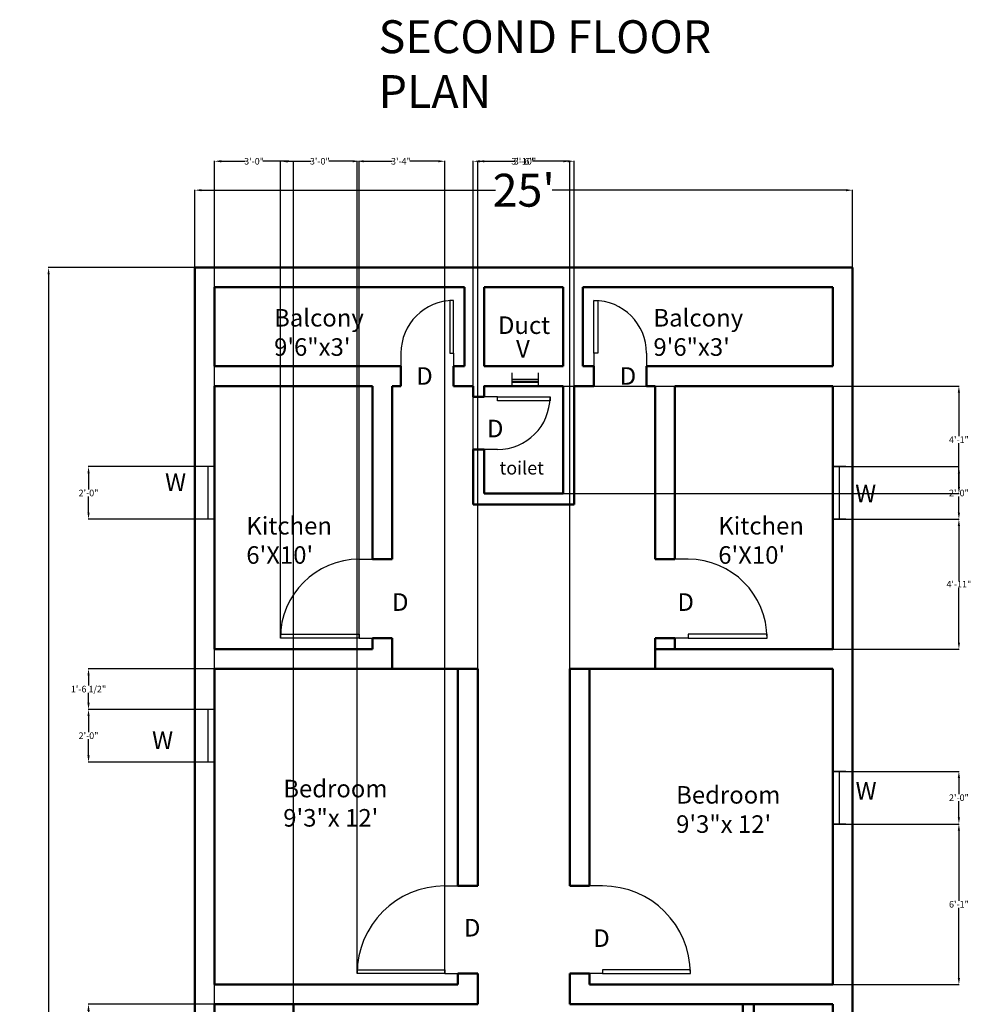
# Model space of a CAD drawing. Units: inches. Extents: x -250 to 2650, y 180 to 1183.
# Tile 6 of 10: x 952 to 1386, y 734 to 1183. Entities that reach past the tile are written whole.
import ezdxf

# ---------------------------------------------------------------- set-up
doc = ezdxf.new("R2010")
doc.units = ezdxf.units.IN
doc.header["$MEASUREMENT"] = 0
for name, color, linetype, lineweight in [('A-ANNO-DIMS', 2, 'Continuous', 18), ('A-ANNO-TEXT', 7, 'Continuous', 18), ('A-AREA-IDEN', 3, 'Continuous', 18), ('A-DOOR', 4, 'Continuous', 25), ('A-GLAZ', 3, 'Continuous', 25), ('A-WALL', 7, 'Continuous', 50)]:
    doc.layers.add(name, color=color, linetype=linetype, lineweight=lineweight)
doc.styles.get("Standard").update_dxf_attribs({"font": 'arial.ttf'})
doc.dimstyles.get("Standard").update_dxf_attribs({"dimtxt": 3, "dimasz": 3, "dimexe": 0.18, "dimexo": 0.0625, "dimgap": 0.09, "dimtad": 0, "dimtih": 1, "dimtoh": 1, "dimdec": 0, "dimzin": 0, "dimdsep": 46, "dimlunit": 3, "dimtxsty": 'Standard', "dimcen": 0.09, "dimadec": 0, "dimazin": 0, "dimtfac": 1, "dimtdec": 0, "dimtofl": 0, "dimtmove": 0, "dimatfit": 3, "dimfxl": 1, "dimtolj": 1, "dimtzin": 0, "dimarcsym": 0})

# ---------------------------------------------------------------- blocks, each defined once
blk = doc.blocks.new('*D34')
at = {"layer": 'A-ANNO-DIMS', "color": 0, "lineweight": -2, "transparency": 16777216}
for p, q in [((1031.71, 1070.09), (1031.71, 1105.5)), ((1034.71, 1105.32), (1168.77, 1105.32)), ((1328.71, 1105.32), (1194.66, 1105.32)), ((1331.71, 1070.09), (1331.71, 1105.5))]:
    blk.add_line(p, q, dxfattribs=at)
at = {"layer": 'A-ANNO-DIMS', "color": 0, "transparency": 16777216}
for points in [[(1034.71, 1105.82), (1034.71, 1104.82), (1031.71, 1105.32)], [(1328.71, 1105.82), (1328.71, 1104.82), (1331.71, 1105.32)]]:
    blk.add_solid(points, dxfattribs=at)
at = {"layer": 'Defpoints', "color": 0, "transparency": 16777216}
for p in [(1031.71, 1105.32), (1031.71, 1070.02), (1331.71, 1070.02)]:
    blk.add_point(p, dxfattribs=at)
at = {"layer": 'A-ANNO-DIMS', "color": 0, "transparency": 16777216, "insert": (1181.71, 1105.32), "char_height": 3, "attachment_point": 5}
blk.add_mtext("\\A1;{\\H5x;25'}", dxfattribs=at)
blk = doc.blocks.new('*D35')
at = {"layer": 'A-ANNO-DIMS', "color": 0, "lineweight": -2, "transparency": 16777216}
for p, q in [((1031.65, 1070.02), (964.83, 1070.02)), ((965.01, 1067.02), (965.01, 657.77)), ((965.01, 233.02), (965.01, 642.28)), ((1031.65, 230.02), (964.83, 230.02))]:
    blk.add_line(p, q, dxfattribs=at)
at = {"layer": 'A-ANNO-DIMS', "color": 0, "transparency": 16777216}
for points in [[(964.51, 1067.02), (965.51, 1067.02), (965.01, 1070.02)], [(964.51, 233.02), (965.51, 233.02), (965.01, 230.02)]]:
    blk.add_solid(points, dxfattribs=at)
at = {"layer": 'Defpoints', "color": 0, "transparency": 16777216}
for p in [(1031.71, 1070.02), (965.01, 230.02), (1031.71, 230.02)]:
    blk.add_point(p, dxfattribs=at)
at = {"layer": 'A-ANNO-DIMS', "color": 0, "transparency": 16777216, "insert": (965.01, 650.02), "char_height": 3, "attachment_point": 5}
blk.add_mtext("\\A1;{\\H5x;70'}", dxfattribs=at)
blk = doc.blocks.new('*U17')
for p, q in [((-24, 0), (-24, -6)), ((0, 0), (0, -6))]:
    blk.add_line(p, q)
blk.add_lwpolyline([(0, 0), (0, 24), (-1.75, 24), (-1.75, 0)], close=True)
blk.add_arc((0, 0), 24, 90, 180)
blk = doc.blocks.new('*U18')
for p, q in [((0, 0), (0, -6)), ((24, 0), (24, -6))]:
    blk.add_line(p, q)
blk.add_lwpolyline([(0, 0), (0, 24), (1.75, 24), (1.75, 0)], close=True)
blk.add_arc((0, 0), 24, 0, 90)
blk = doc.blocks.new('*U19')
for p, q in [((0, 0), (0, -6)), ((24, 0), (24, -6))]:
    blk.add_line(p, q)
blk.add_lwpolyline([(0, 0), (0, 24), (1.75, 24), (1.75, 0)], close=True)
blk.add_arc((0, 0), 24, 0, 90)
blk = doc.blocks.new('*U20')
for p, q in [((-36, 0), (-36, -6)), ((0, 0), (0, -6))]:
    blk.add_line(p, q)
blk.add_lwpolyline([(0, 0), (0, 36), (-1.75, 36), (-1.75, 0)], close=True)
blk.add_arc((0, 0), 36, 90, 180)
blk = doc.blocks.new('*U21')
for p, q in [((-36, 0), (-36, 6)), ((0, 0), (0, 6))]:
    blk.add_line(p, q)
blk.add_lwpolyline([(0, 0), (0, -36), (-1.75, -36), (-1.75, 0)], close=True)
blk.add_arc((0, 0), 36, 180, 270)
blk = doc.blocks.new('*U24')
for p, q in [((-24, 6), (-24, 0)), ((0, 6), (0, 0)), ((0, 3), (-24, 3))]:
    blk.add_line(p, q)
blk = doc.blocks.new('*U23')
for p, q in [((-24, 6), (-24, 0)), ((0, 6), (0, 0)), ((0, 3), (-24, 3))]:
    blk.add_line(p, q)
blk = doc.blocks.new('*U22')
for p, q in [((0, 6), (0, 0)), ((12, 6), (12, 0)), ((0, 3), (12, 3))]:
    blk.add_line(p, q)
blk = doc.blocks.new('*U25')
for p, q in [((-40, 0), (-40, 6)), ((0, 0), (0, 6))]:
    blk.add_line(p, q)
blk.add_lwpolyline([(0, 0), (0, -40), (-1.75, -40), (-1.75, 0)], close=True)
blk.add_arc((0, 0), 40, 180, 270)
blk = doc.blocks.new('*U26')
for p, q in [((-40, 0), (-40, -6)), ((0, 0), (0, -6))]:
    blk.add_line(p, q)
blk.add_lwpolyline([(0, 0), (0, 40), (-1.75, 40), (-1.75, 0)], close=True)
blk.add_arc((0, 0), 40, 90, 180)
blk = doc.blocks.new('*D112')
at = {"layer": 'A-ANNO-DIMS', "color": 0, "lineweight": -2, "transparency": 16777216}
for p, q in [((1040.71, 734.09), (1040.71, 1118.7)), ((1043.71, 1118.52), (1054.64, 1118.52)), ((1073.71, 1118.52), (1062.79, 1118.52)), ((1076.71, 734.09), (1076.71, 1118.7))]:
    blk.add_line(p, q, dxfattribs=at)
at = {"layer": 'A-ANNO-DIMS', "color": 0, "transparency": 16777216}
for points in [[(1043.71, 1119.02), (1043.71, 1118.02), (1040.71, 1118.52)], [(1073.71, 1119.02), (1073.71, 1118.02), (1076.71, 1118.52)]]:
    blk.add_solid(points, dxfattribs=at)
at = {"layer": 'Defpoints', "color": 0, "transparency": 16777216}
for p in [(1076.71, 1118.52), (1040.71, 734.02), (1076.71, 734.02)]:
    blk.add_point(p, dxfattribs=at)
at = {"layer": 'A-ANNO-DIMS', "color": 0, "transparency": 16777216, "insert": (1058.71, 1118.52), "char_height": 3, "attachment_point": 5}
blk.add_mtext('\\A1;3\'-0"', dxfattribs=at)
blk = doc.blocks.new('*D114')
at = {"layer": 'A-ANNO-DIMS', "color": 0, "lineweight": -2, "transparency": 16777216}
for p, q in [((1040.65, 734.02), (983.03, 734.02)), ((983.21, 731.02), (983.21, 717.09)), ((983.21, 699.91), (983.21, 713.84)), ((1040.65, 696.91), (983.03, 696.91))]:
    blk.add_line(p, q, dxfattribs=at)
at = {"layer": 'A-ANNO-DIMS', "color": 0, "transparency": 16777216}
for points in [[(982.71, 731.02), (983.71, 731.02), (983.21, 734.02)], [(982.71, 699.91), (983.71, 699.91), (983.21, 696.91)]]:
    blk.add_solid(points, dxfattribs=at)
at = {"layer": 'Defpoints', "color": 0, "transparency": 16777216}
for p in [(983.21, 734.02), (1040.71, 734.02), (1040.71, 696.91)]:
    blk.add_point(p, dxfattribs=at)
at = {"layer": 'A-ANNO-DIMS', "color": 0, "transparency": 16777216, "insert": (983.21, 715.47), "char_height": 3, "attachment_point": 5}
blk.add_mtext('\\A1;3\'-1"', dxfattribs=at)
blk = doc.blocks.new('*D122')
at = {"layer": 'A-ANNO-DIMS', "color": 0, "lineweight": -2, "transparency": 16777216}
for p, q in [((1160.71, 887.09), (1160.71, 1118.7)), ((1163.71, 1118.52), (1177.64, 1118.52)), ((1199.71, 1118.52), (1185.79, 1118.52)), ((1202.71, 887.09), (1202.71, 1118.7))]:
    blk.add_line(p, q, dxfattribs=at)
at = {"layer": 'A-ANNO-DIMS', "color": 0, "transparency": 16777216}
for points in [[(1163.71, 1119.02), (1163.71, 1118.02), (1160.71, 1118.52)], [(1199.71, 1119.02), (1199.71, 1118.02), (1202.71, 1118.52)]]:
    blk.add_solid(points, dxfattribs=at)
at = {"layer": 'Defpoints', "color": 0, "transparency": 16777216}
for p in [(1202.71, 1118.52), (1160.71, 887.02), (1202.71, 887.02)]:
    blk.add_point(p, dxfattribs=at)
at = {"layer": 'A-ANNO-DIMS', "color": 0, "transparency": 16777216, "insert": (1181.71, 1118.52), "char_height": 3, "attachment_point": 5}
blk.add_mtext('\\A1;3\'-6"', dxfattribs=at)
blk = doc.blocks.new('*D123')
at = {"layer": 'A-ANNO-DIMS', "color": 0, "lineweight": -2, "transparency": 16777216}
for p, q in [((1158.71, 962.09), (1158.71, 1118.7)), ((1161.71, 1118.52), (1176.47, 1118.52)), ((1201.71, 1118.52), (1186.96, 1118.52)), ((1204.71, 962.09), (1204.71, 1118.7))]:
    blk.add_line(p, q, dxfattribs=at)
at = {"layer": 'A-ANNO-DIMS', "color": 0, "transparency": 16777216}
for points in [[(1161.71, 1119.02), (1161.71, 1118.02), (1158.71, 1118.52)], [(1201.71, 1119.02), (1201.71, 1118.02), (1204.71, 1118.52)]]:
    blk.add_solid(points, dxfattribs=at)
at = {"layer": 'Defpoints', "color": 0, "transparency": 16777216}
for p in [(1204.71, 1118.52), (1158.71, 962.02), (1204.71, 962.02)]:
    blk.add_point(p, dxfattribs=at)
at = {"layer": 'A-ANNO-DIMS', "color": 0, "transparency": 16777216, "insert": (1181.71, 1118.52), "char_height": 3, "attachment_point": 5}
blk.add_mtext('\\A1;3\'-10"', dxfattribs=at)
blk = doc.blocks.new('*D124')
at = {"layer": 'A-ANNO-DIMS', "color": 0, "lineweight": -2, "transparency": 16777216}
for p, q in [((1199.78, 1016.02), (1380.39, 1016.02)), ((1380.21, 1013.02), (1380.21, 993.12)), ((1380.21, 970.02), (1380.21, 989.93)), ((1199.78, 967.02), (1380.39, 967.02))]:
    blk.add_line(p, q, dxfattribs=at)
at = {"layer": 'A-ANNO-DIMS', "color": 0, "transparency": 16777216}
for points in [[(1379.71, 1013.02), (1380.71, 1013.02), (1380.21, 1016.02)], [(1379.71, 970.02), (1380.71, 970.02), (1380.21, 967.02)]]:
    blk.add_solid(points, dxfattribs=at)
at = {"layer": 'Defpoints', "color": 0, "transparency": 16777216}
for p in [(1199.71, 1016.02), (1199.71, 967.02), (1380.21, 967.02)]:
    blk.add_point(p, dxfattribs=at)
at = {"layer": 'A-ANNO-DIMS', "color": 0, "transparency": 16777216, "insert": (1380.21, 991.52), "char_height": 3, "attachment_point": 5}
blk.add_mtext('\\A1;4\'-1"', dxfattribs=at)
blk = doc.blocks.new('*D125')
at = {"layer": 'A-ANNO-DIMS', "color": 0, "lineweight": -2, "transparency": 16777216}
for p, q in [((1322.78, 816.25), (1380.39, 816.25)), ((1380.21, 813.25), (1380.21, 781.26)), ((1380.21, 746.02), (1380.21, 778.01)), ((1322.78, 743.02), (1380.39, 743.02))]:
    blk.add_line(p, q, dxfattribs=at)
at = {"layer": 'A-ANNO-DIMS', "color": 0, "transparency": 16777216}
for points in [[(1379.71, 813.25), (1380.71, 813.25), (1380.21, 816.25)], [(1379.71, 746.02), (1380.71, 746.02), (1380.21, 743.02)]]:
    blk.add_solid(points, dxfattribs=at)
at = {"layer": 'Defpoints', "color": 0, "transparency": 16777216}
for p in [(1322.71, 816.25), (1380.21, 816.25), (1322.71, 743.02)]:
    blk.add_point(p, dxfattribs=at)
at = {"layer": 'A-ANNO-DIMS', "color": 0, "transparency": 16777216, "insert": (1380.21, 779.64), "char_height": 3, "attachment_point": 5}
blk.add_mtext('\\A1;6\'-1"', dxfattribs=at)
blk = doc.blocks.new('*D126')
at = {"layer": 'A-ANNO-DIMS', "color": 0, "lineweight": -2, "transparency": 16777216}
for p, q in [((1322.78, 840.25), (1380.39, 840.25)), ((1380.21, 837.25), (1380.21, 829.87)), ((1380.21, 819.25), (1380.21, 826.63)), ((1322.78, 816.25), (1380.39, 816.25))]:
    blk.add_line(p, q, dxfattribs=at)
at = {"layer": 'A-ANNO-DIMS', "color": 0, "transparency": 16777216}
for points in [[(1379.71, 837.25), (1380.71, 837.25), (1380.21, 840.25)], [(1379.71, 819.25), (1380.71, 819.25), (1380.21, 816.25)]]:
    blk.add_solid(points, dxfattribs=at)
at = {"layer": 'Defpoints', "color": 0, "transparency": 16777216}
for p in [(1322.71, 840.25), (1380.21, 840.25), (1322.71, 816.25)]:
    blk.add_point(p, dxfattribs=at)
at = {"layer": 'A-ANNO-DIMS', "color": 0, "transparency": 16777216, "insert": (1380.21, 828.25), "char_height": 3, "attachment_point": 5}
blk.add_mtext('\\A1;2\'-0"', dxfattribs=at)
blk = doc.blocks.new('*D127')
at = {"layer": 'A-ANNO-DIMS', "color": 0, "lineweight": -2, "transparency": 16777216}
for p, q in [((1322.78, 955.23), (1380.39, 955.23)), ((1380.21, 952.23), (1380.21, 927.22)), ((1380.21, 899.02), (1380.21, 924.03)), ((1322.78, 896.02), (1380.39, 896.02))]:
    blk.add_line(p, q, dxfattribs=at)
at = {"layer": 'A-ANNO-DIMS', "color": 0, "transparency": 16777216}
for points in [[(1379.71, 952.23), (1380.71, 952.23), (1380.21, 955.23)], [(1379.71, 899.02), (1380.71, 899.02), (1380.21, 896.02)]]:
    blk.add_solid(points, dxfattribs=at)
at = {"layer": 'Defpoints', "color": 0, "transparency": 16777216}
for p in [(1322.71, 955.23), (1380.21, 955.23), (1322.71, 896.02)]:
    blk.add_point(p, dxfattribs=at)
at = {"layer": 'A-ANNO-DIMS', "color": 0, "transparency": 16777216, "insert": (1380.21, 925.63), "char_height": 3, "attachment_point": 5}
blk.add_mtext('\\A1;4\'-11"', dxfattribs=at)
blk = doc.blocks.new('*D128')
at = {"layer": 'A-ANNO-DIMS', "color": 0, "lineweight": -2, "transparency": 16777216}
for p, q in [((1322.78, 979.23), (1380.39, 979.23)), ((1380.21, 976.23), (1380.21, 968.85)), ((1380.21, 958.23), (1380.21, 965.61)), ((1322.78, 955.23), (1380.39, 955.23))]:
    blk.add_line(p, q, dxfattribs=at)
at = {"layer": 'A-ANNO-DIMS', "color": 0, "transparency": 16777216}
for points in [[(1379.71, 976.23), (1380.71, 976.23), (1380.21, 979.23)], [(1379.71, 958.23), (1380.71, 958.23), (1380.21, 955.23)]]:
    blk.add_solid(points, dxfattribs=at)
at = {"layer": 'Defpoints', "color": 0, "transparency": 16777216}
for p in [(1322.71, 979.23), (1380.21, 979.23), (1322.71, 955.23)]:
    blk.add_point(p, dxfattribs=at)
at = {"layer": 'A-ANNO-DIMS', "color": 0, "transparency": 16777216, "insert": (1380.21, 967.23), "char_height": 3, "attachment_point": 5}
blk.add_mtext('\\A1;2\'-0"', dxfattribs=at)
blk = doc.blocks.new('*D129')
at = {"layer": 'A-ANNO-DIMS', "color": 0, "lineweight": -2, "transparency": 16777216}
for p, q in [((1040.65, 868.53), (983.03, 868.53)), ((983.21, 865.53), (983.21, 858.15)), ((983.21, 847.53), (983.21, 854.91)), ((1040.65, 844.53), (983.03, 844.53))]:
    blk.add_line(p, q, dxfattribs=at)
at = {"layer": 'A-ANNO-DIMS', "color": 0, "transparency": 16777216}
for points in [[(982.71, 865.53), (983.71, 865.53), (983.21, 868.53)], [(982.71, 847.53), (983.71, 847.53), (983.21, 844.53)]]:
    blk.add_solid(points, dxfattribs=at)
at = {"layer": 'Defpoints', "color": 0, "transparency": 16777216}
for p in [(983.21, 868.53), (1040.71, 868.53), (1040.71, 844.53)]:
    blk.add_point(p, dxfattribs=at)
at = {"layer": 'A-ANNO-DIMS', "color": 0, "transparency": 16777216, "insert": (983.21, 856.53), "char_height": 3, "attachment_point": 5}
blk.add_mtext('\\A1;2\'-0"', dxfattribs=at)
blk = doc.blocks.new('*D130')
at = {"layer": 'A-ANNO-DIMS', "color": 0, "lineweight": -2, "transparency": 16777216}
for p, q in [((1040.65, 887.02), (983.03, 887.02)), ((983.21, 884.02), (983.21, 879.42)), ((983.21, 871.53), (983.21, 876.14)), ((1040.65, 868.53), (983.03, 868.53))]:
    blk.add_line(p, q, dxfattribs=at)
at = {"layer": 'A-ANNO-DIMS', "color": 0, "transparency": 16777216}
for points in [[(982.71, 884.02), (983.71, 884.02), (983.21, 887.02)], [(982.71, 871.53), (983.71, 871.53), (983.21, 868.53)]]:
    blk.add_solid(points, dxfattribs=at)
at = {"layer": 'Defpoints', "color": 0, "transparency": 16777216}
for p in [(983.21, 887.02), (1040.71, 887.02), (1040.71, 868.53)]:
    blk.add_point(p, dxfattribs=at)
at = {"layer": 'A-ANNO-DIMS', "color": 0, "transparency": 16777216, "insert": (983.21, 877.78), "char_height": 3, "attachment_point": 5}
blk.add_mtext('\\A1;1\'-6 1/2"', dxfattribs=at)
blk = doc.blocks.new('*D131')
at = {"layer": 'A-ANNO-DIMS', "color": 0, "lineweight": -2, "transparency": 16777216}
for p, q in [((1040.65, 979.23), (983.03, 979.23)), ((983.21, 976.23), (983.21, 968.85)), ((983.21, 958.23), (983.21, 965.61)), ((1040.65, 955.23), (983.03, 955.23))]:
    blk.add_line(p, q, dxfattribs=at)
at = {"layer": 'A-ANNO-DIMS', "color": 0, "transparency": 16777216}
for points in [[(982.71, 976.23), (983.71, 976.23), (983.21, 979.23)], [(982.71, 958.23), (983.71, 958.23), (983.21, 955.23)]]:
    blk.add_solid(points, dxfattribs=at)
at = {"layer": 'Defpoints', "color": 0, "transparency": 16777216}
for p in [(983.21, 979.23), (1040.71, 979.23), (1040.71, 955.23)]:
    blk.add_point(p, dxfattribs=at)
at = {"layer": 'A-ANNO-DIMS', "color": 0, "transparency": 16777216, "insert": (983.21, 967.23), "char_height": 3, "attachment_point": 5}
blk.add_mtext('\\A1;2\'-0"', dxfattribs=at)
blk = doc.blocks.new('*D132')
at = {"layer": 'A-ANNO-DIMS', "color": 0, "lineweight": -2, "transparency": 16777216}
for p, q in [((1105.71, 748.09), (1105.71, 1118.7)), ((1108.71, 1118.52), (1121.64, 1118.52)), ((1142.71, 1118.52), (1129.79, 1118.52)), ((1145.71, 748.09), (1145.71, 1118.7))]:
    blk.add_line(p, q, dxfattribs=at)
at = {"layer": 'A-ANNO-DIMS', "color": 0, "transparency": 16777216}
for points in [[(1108.71, 1119.02), (1108.71, 1118.02), (1105.71, 1118.52)], [(1142.71, 1119.02), (1142.71, 1118.02), (1145.71, 1118.52)]]:
    blk.add_solid(points, dxfattribs=at)
at = {"layer": 'Defpoints', "color": 0, "transparency": 16777216}
for p in [(1145.71, 1118.52), (1105.71, 748.02), (1145.71, 748.02)]:
    blk.add_point(p, dxfattribs=at)
at = {"layer": 'A-ANNO-DIMS', "color": 0, "transparency": 16777216, "insert": (1125.71, 1118.52), "char_height": 3, "attachment_point": 5}
blk.add_mtext('\\A1;3\'-4"', dxfattribs=at)
blk = doc.blocks.new('*D133')
at = {"layer": 'A-ANNO-DIMS', "color": 0, "lineweight": -2, "transparency": 16777216}
for p, q in [((1070.71, 901.09), (1070.71, 1118.7)), ((1073.71, 1118.52), (1084.64, 1118.52)), ((1103.71, 1118.52), (1092.79, 1118.52)), ((1106.71, 901.09), (1106.71, 1118.7))]:
    blk.add_line(p, q, dxfattribs=at)
at = {"layer": 'A-ANNO-DIMS', "color": 0, "transparency": 16777216}
for points in [[(1073.71, 1119.02), (1073.71, 1118.02), (1070.71, 1118.52)], [(1103.71, 1119.02), (1103.71, 1118.02), (1106.71, 1118.52)]]:
    blk.add_solid(points, dxfattribs=at)
at = {"layer": 'Defpoints', "color": 0, "transparency": 16777216}
for p in [(1106.71, 1118.52), (1070.71, 901.02), (1106.71, 901.02)]:
    blk.add_point(p, dxfattribs=at)
at = {"layer": 'A-ANNO-DIMS', "color": 0, "transparency": 16777216, "insert": (1088.71, 1118.52), "char_height": 3, "attachment_point": 5}
blk.add_mtext('\\A1;3\'-0"', dxfattribs=at)

msp = doc.modelspace()

# ---------------------------------------------------------------- linework, layer by layer
at = {"layer": 'A-WALL'}
for p, q in [((1331.71, 1070.02), (1031.71, 1070.02)), ((1031.71, 1070.02), (1031.71, 230.02)), ((1331.71, 230.02), (1331.71, 1070.02)), ((1154.71, 1061.02), (1040.71, 1061.02)), ((1040.71, 1061.02), (1040.71, 1025.02)), ((1154.71, 1061.02), (1154.71, 1025.02)), ((1199.71, 1061.02), (1163.71, 1061.02)), ((1163.71, 1061.02), (1163.71, 1025.02)), ((1199.71, 1025.02), (1199.71, 1061.02)), ((1208.71, 1025.02), (1208.71, 1061.02)), ((1322.71, 1061.02), (1208.71, 1061.02)), ((1322.71, 1025.02), (1322.71, 1061.02)), ((1322.71, 1025.02), (1322.71, 1061.02)), ((1322.71, 1025.02), (1322.71, 1061.02)), ((1322.71, 1025.02), (1322.71, 1061.02)), ((1125.71, 1025.02), (1040.71, 1025.02)), ((1125.71, 1025.02), (1125.71, 1016.02)), ((1154.71, 1025.02), (1149.71, 1025.02)), ((1149.71, 1016.02), (1149.71, 1025.02)), ((1199.71, 1025.02), (1163.71, 1025.02)), ((1213.71, 1025.02), (1208.71, 1025.02)), ((1213.71, 1016.02), (1213.71, 1025.02)), ((1322.71, 1025.02), (1237.71, 1025.02)), ((1237.71, 1025.02), (1237.71, 1016.02)), ((1112.71, 1016.02), (1040.71, 1016.02)), ((1040.71, 1016.02), (1040.71, 896.02)), ((1112.71, 1016.02), (1112.71, 937.02)), ((1125.71, 1016.02), (1121.71, 1016.02)), ((1121.71, 1016.02), (1121.71, 937.02)), ((1158.71, 1016.02), (1149.71, 1016.02)), ((1158.71, 1016.02), (1158.71, 1011.02)), ((1163.71, 1016.03), (1163.71, 1011.02)), ((1199.71, 1016.02), (1163.71, 1016.02)), ((1188.4, 1017.95), (1176.4, 1017.95)), ((1199.71, 967.02), (1199.71, 1016.02)), ((1204.71, 962.02), (1204.71, 1016.02)), ((1213.71, 1016.02), (1204.71, 1016.02)), ((1241.71, 1016.02), (1237.71, 1016.02)), ((1241.71, 937.02), (1241.71, 1016.02)), ((1250.71, 937.02), (1250.71, 1016.02)), ((1322.71, 1016.02), (1250.71, 1016.02)), ((1322.71, 896.02), (1322.71, 1016.02)), ((1322.71, 896.02), (1322.71, 1016.02)), ((1322.71, 896.02), (1322.71, 1016.02)), ((1163.71, 1011.02), (1158.71, 1011.02)), ((1158.71, 987.02), (1158.71, 962.02)), ((1163.71, 987.02), (1158.71, 987.02)), ((1163.71, 987.02), (1163.71, 967.02)), ((1199.71, 967.02), (1163.71, 967.02)), ((1204.71, 962.02), (1158.71, 962.02)), ((1112.71, 937.02), (1121.71, 937.02)), ((1250.71, 937.02), (1241.71, 937.02)), ((1112.71, 901.02), (1112.71, 896.02)), ((1112.71, 901.02), (1121.71, 901.02)), ((1121.71, 901.02), (1121.71, 887.02)), ((1241.71, 887.02), (1241.71, 901.02)), ((1250.71, 901.02), (1241.71, 901.02)), ((1250.71, 896.02), (1250.71, 901.02)), ((1112.71, 896.02), (1040.71, 896.02)), ((1322.71, 896.02), (1241.71, 896.02)), ((1160.71, 887.02), (1040.71, 887.02)), ((1040.71, 887.02), (1040.71, 743.02)), ((1151.71, 887.02), (1151.71, 788.02)), ((1160.71, 887.02), (1160.71, 788.02)), ((1202.71, 788.02), (1202.71, 887.02)), ((1322.71, 887.02), (1202.71, 887.02)), ((1211.71, 788.02), (1211.71, 887.02)), ((1322.71, 743.02), (1322.71, 887.02)), ((1322.71, 743.02), (1322.71, 887.02)), ((1322.71, 743.02), (1322.71, 887.02)), ((1151.71, 788.02), (1160.71, 788.02)), ((1211.71, 788.02), (1202.71, 788.02)), ((1151.71, 748.02), (1151.71, 743.02)), ((1151.71, 748.02), (1160.71, 748.02)), ((1160.71, 748.02), (1160.71, 734.02)), ((1211.71, 748.02), (1202.71, 748.02)), ((1202.71, 748.02), (1202.71, 734.02)), ((1211.71, 743.02), (1211.71, 748.02)), ((1151.71, 743.02), (1040.71, 743.02)), ((1322.71, 743.02), (1211.71, 743.02)), ((1160.71, 734.02), (1040.71, 734.02)), ((1040.71, 734.02), (1040.71, 696.91)), ((1076.71, 696.91), (1076.71, 734.02)), ((1322.71, 734.02), (1202.71, 734.02)), ((1281.71, 686.91), (1281.71, 734.02)), ((1281.71, 686.91), (1281.71, 734.02)), ((1286.71, 696.91), (1286.71, 734.02)), ((1322.71, 696.91), (1322.71, 734.02)), ((1322.71, 716.02), (1322.71, 734.02))]:
    msp.add_line(p, q, dxfattribs=at)

# ---------------------------------------------------------------- block references
at = {"layer": 'A-DOOR'}
for name, p in [('*U17', (1149.71, 1031.02)), ('*U18', (1213.71, 1031.02))]:
    msp.add_blockref(name, p, dxfattribs=at)
at = {"layer": 'A-DOOR', "rotation": 270}
for name, p in [('*U19', (1169.71, 1011.02)), ('*U21', (1106.71, 901.02)), ('*U20', (1256.71, 901.02)), ('*U25', (1145.71, 748.02)), ('*U26', (1217.71, 748.02))]:
    msp.add_blockref(name, p, dxfattribs=at)
at = {"layer": 'A-GLAZ'}
for name, p, rotation in [('*U22', (1188.4, 1021.95), 180), ('*U23', (1034.71, 955.23), 270), ('*U24', (1322.71, 955.23), 270), ('*U23', (1034.71, 844.53), 270), ('*U24', (1322.71, 816.25), 270)]:
    msp.add_blockref(name, p, dxfattribs=dict(at, rotation=rotation))

# ---------------------------------------------------------------- texts
at = {"layer": 'A-ANNO-TEXT', "attachment_point": 1}
for s, width, insert, char_height in [('SECOND FLOOR PLAN ', 207.4062, (1115.52, 1182.82), 15), ('V', 10.3916, (1178.22, 1036.98), 8), ('D', 10.3916, (1132.7, 1024.6), 8), ('D', 10.3916, (1225.51, 1024.6), 8), ('D', 10.3916, (1164.95, 1000.62), 8), ('W', 10.3916, (1018.13, 976.14), 8), ('W', 10.3916, (1332.9, 971.03), 8), ('D', 10.3916, (1121.66, 921.46), 8), ('D', 10.3916, (1251.84, 921.46), 8), ('W', 10.3916, (1012.2, 858.45), 8), ('W', 10.3916, (1333.08, 835.41), 8), ('D', 10.3916, (1154.45, 772.95), 8), ('D', 10.3916, (1213.44, 768.2), 8)]:
    msp.add_mtext_dynamic_manual_height_columns(s, width=width, gutter_width=1, heights=[0], dxfattribs=dict(at, insert=insert, char_height=char_height))
at = {"layer": 'A-AREA-IDEN', "attachment_point": 1}
for s, width, heights, insert, char_height in [('Balcony 9\'6"x3\'', 37.1044, [0], (1067.85, 1051.13), 8), ('Balcony 9\'6"x3\'', 37.1044, [0], (1240.87, 1051.13), 8), ('{\\H2.66667x;Duct} ', 7.71, [3.05], (1169.97, 1047.76), 3), ('toilet', 19.3499, [0], (1170.68, 981.65), 6), ("Kitchen 6'X10'", 37.1044, [0], (1055.18, 956.28), 8), ("Kitchen 6'X10'", 37.1044, [0], (1270.45, 956.28), 8), ('Bedroom \\P9\'3"x 12\'', 51.3886, [0], (1072.03, 836.41), 8), ('Bedroom \\P9\'3"x 12\'', 51.3886, [0], (1251.23, 833.56), 8)]:
    msp.add_mtext_dynamic_manual_height_columns(s, width=width, gutter_width=1, heights=heights, dxfattribs=dict(at, insert=insert, char_height=char_height))

# ---------------------------------------------------------------- dimensions: what is measured, and where the dimension line sits
at = {"layer": 'A-ANNO-DIMS'}
for base, p1, p2, picture, middle in [((1076.71, 1118.52), (1040.71, 734.02), (1076.71, 734.02), '*D112', (1058.71, 1118.52)), ((1106.71, 1118.52), (1070.71, 901.02), (1106.71, 901.02), '*D133', (1088.71, 1118.52)), ((1145.71, 1118.52), (1105.71, 748.02), (1145.71, 748.02), '*D132', (1125.71, 1118.52)), ((1204.71, 1118.52), (1158.71, 962.02), (1204.71, 962.02), '*D123', (1181.71, 1118.52)), ((1202.71, 1118.52), (1160.71, 887.02), (1202.71, 887.02), '*D122', (1181.71, 1118.52))]:
    dim = msp.add_linear_dim(base=base, p1=p1, p2=p2, dimstyle='Standard', override={"dimdec": 1, "dimlfac": 1, "dimrnd": 0, "dimzin": 1, "dimdsep": 46, "dimlunit": 4, "dimfrac": 2}, dxfattribs=at)
    dim.commit()
    dim.dimension.update_dxf_attribs({"geometry": picture, "text_midpoint": middle})
dim = msp.add_linear_dim(base=(1031.71, 1105.32), p1=(1331.71, 1070.02), p2=(1031.71, 1070.02), text='{\\H5x;<>}', dimstyle='Standard', override={"dimclrd": 0, "dimclre": 0, "dimclrt": 0}, dxfattribs=at)
dim.commit()
dim.dimension.update_dxf_attribs({"geometry": '*D34', "text_midpoint": (1181.71, 1105.32)})
dim = msp.add_linear_dim(base=(965.01, 230.02), p1=(1031.71, 1070.02), p2=(1031.71, 230.02), angle=90, text='{\\H5x;<>}', dimstyle='Standard', override={"dimclrd": 0, "dimclre": 0, "dimclrt": 0}, dxfattribs=at)
dim.commit()
dim.dimension.update_dxf_attribs({"geometry": '*D35', "text_midpoint": (965.01, 650.02)})
for base, p1, p2, picture, middle in [((1380.21, 967.02), (1199.71, 1016.02), (1199.71, 967.02), '*D124', (1380.21, 991.52)), ((983.21, 979.23), (1040.71, 955.23), (1040.71, 979.23), '*D131', (983.21, 967.23)), ((1380.21, 979.23), (1322.71, 955.23), (1322.71, 979.23), '*D128', (1380.21, 967.23)), ((1380.21, 955.23), (1322.71, 896.02), (1322.71, 955.23), '*D127', (1380.21, 925.63)), ((983.21, 887.02), (1040.71, 868.53), (1040.71, 887.02), '*D130', (983.21, 877.78)), ((983.21, 868.53), (1040.71, 844.53), (1040.71, 868.53), '*D129', (983.21, 856.53)), ((1380.21, 840.25), (1322.71, 816.25), (1322.71, 840.25), '*D126', (1380.21, 828.25)), ((1380.21, 816.25), (1322.71, 743.02), (1322.71, 816.25), '*D125', (1380.21, 779.64)), ((983.21, 734.02), (1040.71, 696.91), (1040.71, 734.02), '*D114', (983.21, 715.47))]:
    dim = msp.add_linear_dim(base=base, p1=p1, p2=p2, angle=90, dimstyle='Standard', override={"dimdec": 1, "dimlfac": 1, "dimrnd": 0, "dimzin": 1, "dimdsep": 46, "dimlunit": 4, "dimfrac": 2}, dxfattribs=at)
    dim.commit()
    dim.dimension.update_dxf_attribs({"geometry": picture, "text_midpoint": middle})

doc.saveas('drawing.dxf')
